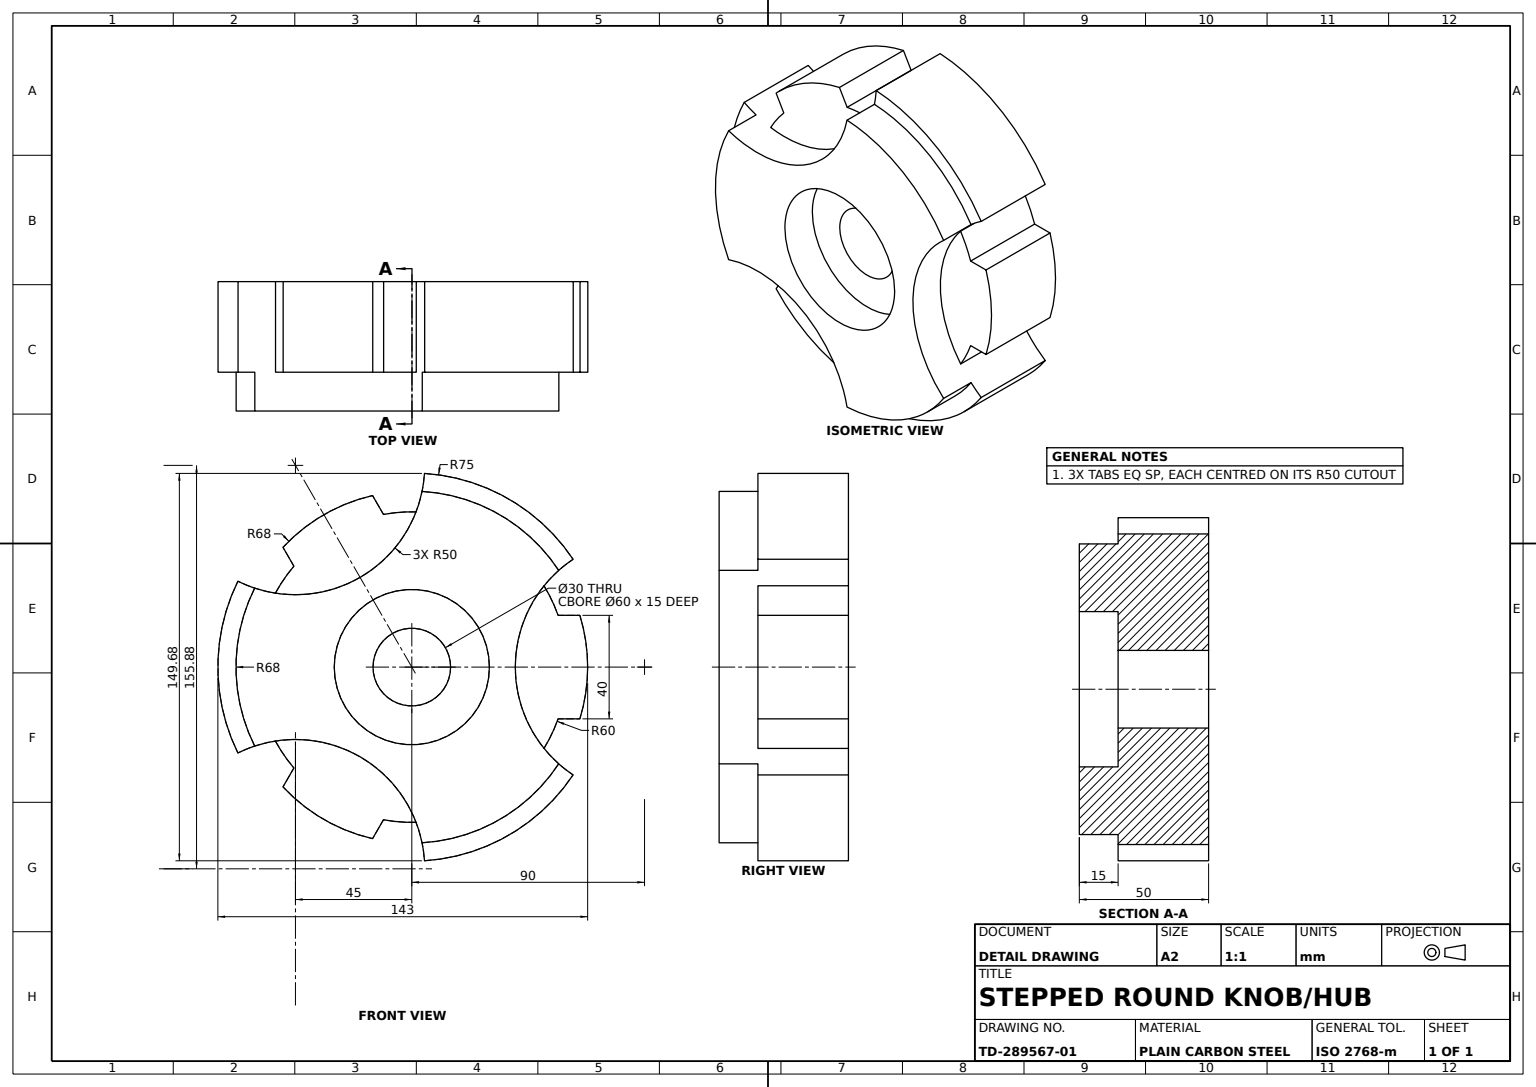
SolidWorks part; units mm, degrees
material "Plain Carbon Steel"
ref_plane "Front Plane" through (0, 0, 0) normal (0, 0, 1) x (1, 0, 0)
ref_plane "Top Plane" through (0, 0, 0) normal (0, 1, 0) x (1, 0, 0)
ref_plane "Right Plane" through (0, 0, 0) normal (1, 0, 0) x (0, 0, -1)
sketch "Base Profile Sketch" plane through (0, 0, 0) normal (0, 1, 0) x (1, 0, 0)
  arc A0 (-41.6664, 62.3611) -> (-74.8395, 4.9036) centre (0, 0) ccw
  arc A2 (74.8395, 4.9036) -> (33.1731, -67.2647) centre (77.9423, -45) ccw
  arc A3 (-33.1731, -67.2647) -> (-74.8395, 4.9036) centre (-77.9423, -45) ccw
  arc A4 (-41.6664, 62.3611) -> (41.6664, 62.3611) centre (0, 90) ccw
  arc A5 (-33.1731, -67.2647) -> (33.1731, -67.2647) centre (0, 0) ccw
  arc A6 (74.8395, 4.9036) -> (41.6664, 62.3611) centre (0, 0) ccw
  dimension "D1" = 150
  dimension "D2" = 77.9423
  dimension "D4" = 100
  dimension "D3" = 45
  dimension "D6" = 90
  dimension "D7" = 155.8846
  dimension "D5" = 3
extrude "Base Body 35mm" add sketch "Base Profile Sketch" along normal blind 35
sketch "Lobe Profile Sketch" plane through (0, 0, 0) normal (0, -1, 0) x (1, 0, 0)
  line L0 (20, -56.5685) -> (20, -64.9923)
  line L1 (-20, -56.5685) -> (-20, -64.9923)
  line L2 (58.9898, 10.9638) -> (66.285, 15.1756)
  line L3 (38.9898, 45.6048) -> (46.285, 49.8167)
  line L4 (-58.9898, 10.9638) -> (-66.285, 15.1756)
  line L5 (-38.9898, 45.6048) -> (-46.285, 49.8167)
  arc A0 (-46.285, 49.8167) -> (-66.285, 15.1756) centre (0, 0) ccw
  arc A1 (38.9898, 45.6048) -> (-38.9898, 45.6048) centre (0, 0) ccw
  arc A2 (-58.9898, 10.9638) -> (-20, -56.5685) centre (0, 0) ccw
  arc A3 (20, -56.5685) -> (58.9898, 10.9638) centre (0, 0) ccw
  arc A4 (-20, -64.9923) -> (20, -64.9923) centre (0, 0) ccw
  arc A5 (66.285, 15.1756) -> (46.285, 49.8167) centre (0, 0) ccw
  point P4 (10, -17.3205)
  point P6 (116.75, 67.4057)
  point P7 (126.75, 50.0851)
  point P8 (-10, 17.3205)
  point P9 (106.75, 84.7262)
  dimension "D1" = 136
  dimension "D2" = 120
  dimension "D3" = 40
  dimension "D4" = 45.6048
  dimension "D5" = 58.9898
  dimension "D6" = 3
extrude "Three-Lobe Profile 35mm" add sketch "Lobe Profile Sketch" against normal blind 35
sketch "Hub Profile Sketch" plane through (0, 35, 0) normal (0, 1, 0) x (1, 0, 0)
  arc A0 (-37.3866, 56.8) -> (-67.8836, 3.9778) centre (0, 0) ccw
  arc A2 (-37.3866, 56.8) -> (37.3866, 56.8) centre (0, 90) ccw
  arc A3 (67.8836, 3.9778) -> (30.4969, -60.7778) centre (77.9423, -45) ccw
  arc A4 (-30.4969, -60.7778) -> (-67.8836, 3.9778) centre (-77.9423, -45) ccw
  arc A5 (-30.4969, -60.7778) -> (30.4969, -60.7778) centre (0, 0) ccw
  arc A6 (67.8836, 3.9778) -> (37.3866, 56.8) centre (0, 0) ccw
  dimension "D1" = 136
  dimension "D2" = 60.7778
  dimension "D3" = 100
  dimension "D5" = 30.4969
  dimension "D6" = 67.8836
  dimension "D4" = 3
extrude "Raised Hub 15mm" add sketch "Hub Profile Sketch" along normal blind 15
sketch "Counterbore Sketch Ø60" plane through (0, 50, 0) normal (0, 1, 0) x (1, 0, 0)
  circle A0 centre (0, 0) radius 30
  dimension "60" = 60
extrude "Counterbore Ø60x15" cut sketch "Counterbore Sketch Ø60" against normal blind 15
sketch "Bore Sketch Ø30" plane through (0, 35, 0) normal (0, 1, 0) x (1, 0, 0)
  circle A0 centre (0, 0) radius 15
  dimension "D1" = 30
extrude "Through Bore Ø30" cut sketch "Bore Sketch Ø30" against normal blind 35
